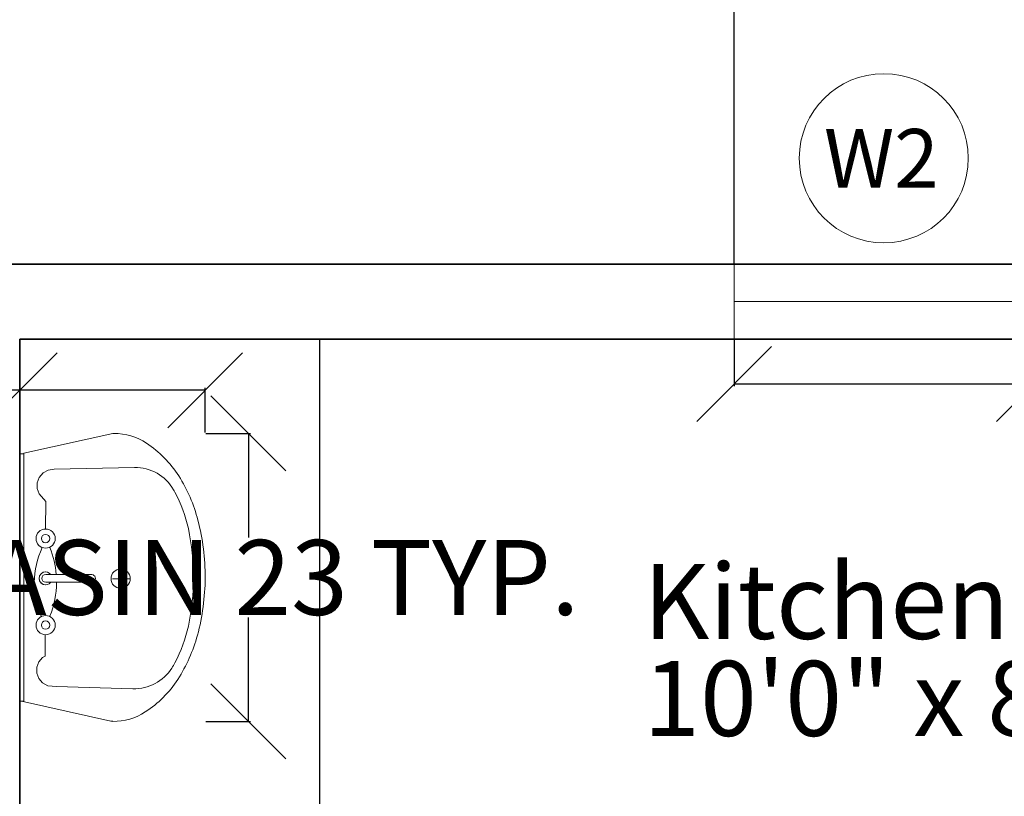
# Model space of a CAD drawing. Units: inches. Extents: x -1198 to -69, y -512 to 437.
# Tile 16 of 50: x -1013 to -934, y 221 to 283. Entities that reach past the tile are written whole.
import ezdxf

# ---------------------------------------------------------------- set-up
doc = ezdxf.new("R2010")
doc.units = ezdxf.units.IN
doc.header["$MEASUREMENT"] = 0
for name, color, linetype, lineweight in [('A-ANNO-DIMS', 2, 'Continuous', 18), ('A-ANNO-SYMB', 7, 'Continuous', 18), ('A-AREA-IDEN', 7, 'Continuous', 18), ('A-FLOR-CASE', 7, 'Continuous', 25), ('A-FLOR-FIXT', 60, 'Continuous', 18), ('A-WALL', 7, 'Continuous', 35), ('windows', 160, 'Continuous', 18)]:
    doc.layers.add(name, color=color, linetype=linetype, lineweight=lineweight)
doc.styles.get("Standard").update_dxf_attribs({"font": 'arial.ttf'})
doc.dimstyles.get("Standard").update_dxf_attribs({"dimtxt": 6, "dimasz": 6, "dimexe": 0.18, "dimexo": 0.0625, "dimgap": 0.09, "dimtad": 0, "dimtih": 1, "dimtoh": 1, "dimdec": 0, "dimzin": 0, "dimdsep": 46, "dimlunit": 4, "dimtxsty": 'Standard', "dimblk": 'OBLIQUE', "dimcen": 0.09, "dimadec": 0, "dimazin": 0, "dimtfac": 1, "dimtdec": 0, "dimtofl": 0, "dimtmove": 0, "dimatfit": 3, "dimfxl": 1, "dimtolj": 1, "dimtzin": 0, "dimarcsym": 0})

# ---------------------------------------------------------------- blocks, each defined once
blk = doc.blocks.new('A$C6AA41FE3')
at = {"linetype": 'ByBlock'}
for p, q in [((0.1919, 0.5849), (0.3733, 0.5439)), ((0.3687, 0.04), (0.3687, 0.5439)), ((0.3687, 0.5439), (0.3772, 0.5439)), ((0.3772, 0.0411), (0.3772, 0.5439)), ((0.3026, 0.514), (0.1469, 0.5187)), ((0.32, 0.5127), (0.3026, 0.514)), ((0.3305, 0.5069), (0.32, 0.5127)), ((0.3383, 0.4979), (0.3305, 0.5069)), ((0.3425, 0.4869), (0.3383, 0.4979)), ((0.3425, 0.4752), (0.3425, 0.4869)), ((0.3305, 0.4553), (0.3383, 0.4642)), ((0.3383, 0.4642), (0.3425, 0.4752)), ((0.3251, 0.409), (0.3253, 0.4524)), ((0.3253, 0.4524), (0.3305, 0.4553)), ((0.1747, 0.3146), (0.1747, 0.2774)), ((0.2326, 0.3025), (0.3243, 0.3025)), ((0.2326, 0.3021), (0.2326, 0.3025)), ((0.3243, 0.3025), (0.3243, 0.3024)), ((0.1525, 0.2951), (0.1884, 0.2951)), ((0.2326, 0.2863), (0.2326, 0.2867)), ((0.3243, 0.2863), (0.2326, 0.2863)), ((0.3243, 0.2864), (0.3243, 0.2863)), ((0.3243, 0.1379), (0.3245, 0.1941)), ((0.3374, 0.1229), (0.3243, 0.1379)), ((0.3415, 0.1119), (0.3374, 0.1229)), ((0.3374, 0.0892), (0.3415, 0.1002)), ((0.3415, 0.1002), (0.3415, 0.1119)), ((0.3191, 0.0744), (0.3296, 0.0802)), ((0.3296, 0.0802), (0.3374, 0.0892)), ((0.144, 0.0693), (0.3071, 0.0724)), ((0.3071, 0.0724), (0.3191, 0.0744)), ((0.3772, 0.0411), (0.3687, 0.0411)), ((0.188, 0), (0.3687, 0.04))]:
    blk.add_line(p, q, dxfattribs=at)
for centre, radius in [((0.3245, 0.3895), 0.0195), ((0.3245, 0.3895), 0.00849), ((0.172, 0.2951), 0.0195), ((0.3245, 0.2136), 0.0195), ((0.3245, 0.2136), 0.00849)]:
    blk.add_circle(centre, radius, dxfattribs=at)
for centre, radius, start, end in [((0.1864, 0.4671), 0.118, 89.1785, 123.1413), ((0.1877, 0.4667), 0.1183, 87.9266, 89.8113), ((0.241, 0.3799), 0.2208, 122.6461, 147.0936), ((0.1441, 0.4288), 0.09, 88.2595, 147.7588), ((0.3304, 0.324), 0.3262, 147.383, 164.6821), ((0.3272, 0.3256), 0.3003, 152.1306, 167.3001), ((0.2193, 0.3814), 0.1789, 147.7588, 151.7723), ((0.4743, 0.289), 0.4743, 165.1956, 179.4863), ((0.5, 0.2906), 0.4766, 167.7656, 179.7702), ((0.4839, 0.3016), 0.1818, 157.4645, 179.7061), ((0.1798, 0.3042), 0.1678, 334.4875, 24.1794), ((0.2312, 0.2944), 0.0078, 80.1551, 279.8449), ((0.3243, 0.2944), 0.013, 218.4979, 141.5021), ((0.3243, 0.2944), 0.0134, 270, 90), ((0.3243, 0.2944), 0.00798, 270, 90), ((0.4743, 0.2935), 0.4743, 180.0316, 194.3223), ((0.5, 0.2944), 0.4766, 180.2298, 192.2344), ((0.4839, 0.3016), 0.1818, 184.8087, 202.5355), ((0.3272, 0.2594), 0.3003, 192.6999, 207.8694), ((0.33, 0.2597), 0.3262, 194.841, 212.14), ((0.2193, 0.2037), 0.1789, 208.2281, 209.9799), ((0.1423, 0.1592), 0.09, 209.9799, 271.0537), ((0.2402, 0.2046), 0.2208, 212.4413, 236.8887), ((0.1848, 0.1179), 0.1179, 236.4084, 270.3713), ((0.1861, 0.1183), 0.1183, 269.7541, 270.9471)]:
    blk.add_arc(centre, radius, start, end, dxfattribs=at)
blk = doc.blocks.new('A1')
at = {"xscale": 1000, "yscale": 1000, "zscale": 1000, "rotation": 90}
blk.add_blockref('A$C6AA41FE3', (292.5, -377.2), dxfattribs=at)
blk = doc.blocks.new('WIN-W2-24')
at = {"ltscale": 10}
for p, q in [((0, 6), (0, 0)), ((24, 6), (24, 0)), ((0, 3), (24, 3))]:
    blk.add_line(p, q, dxfattribs=at)
blk = doc.blocks.new('COUNTER-L')
at = {"ltscale": 10}
for p, q in [((0, 96), (0, 24)), ((49.349, 24), (0, 24)), ((49.349, 0), (49.349, 24))]:
    blk.add_line(p, q, dxfattribs=at)
blk = doc.blocks.new('TAG-W2')
at = {"ltscale": 10}
blk.add_circle((0, 0), 6.767, dxfattribs=at)
blk.add_text('W2', height=4.6996, dxfattribs=at).set_placement((-4.791, -2.359))
blk = doc.blocks.new('_Oblique')
at = {"color": 0, "linetype": 'ByBlock', "lineweight": -2}
blk.add_line((-0.5, -0.5), (0.5, 0.5), dxfattribs=at)
blk = doc.blocks.new('*D40')
at = {"layer": 'A-ANNO-DIMS', "color": 0, "lineweight": -2, "ltscale": 10, "transparency": 16777216}
for p, q in [((-997.84, 249.671), (-994.265, 249.671)), ((-994.445, 249.671), (-994.445, 241.34)), ((-994.445, 226.62), (-994.445, 234.951)), ((-997.84, 226.62), (-994.265, 226.62))]:
    blk.add_line(p, q, dxfattribs=at)
at = {"layer": 'DEFPOINTS', "color": 0, "ltscale": 10, "transparency": 16777216}
for p in [(-997.902, 249.671), (-994.445, 249.671), (-997.902, 226.62)]:
    blk.add_point(p, dxfattribs=at)
at = {"layer": 'A-ANNO-DIMS', "color": 0, "lineweight": -2, "ltscale": 10, "transparency": 16777216, "xscale": 6, "yscale": 6, "zscale": 6}
for p, rotation in [((-994.445, 249.671), 90), ((-994.445, 226.62), 270)]:
    blk.add_blockref('_Oblique', p, dxfattribs=dict(at, rotation=rotation))
at = {"layer": 'A-ANNO-DIMS', "color": 0, "ltscale": 10, "transparency": 16777216, "insert": (-994.445, 238.145), "char_height": 6, "attachment_point": 5}
blk.add_mtext('\\A1;BASIN 23 TYP.', dxfattribs=at)
blk = doc.blocks.new('*D41')
at = {"layer": 'A-ANNO-DIMS', "color": 0, "lineweight": -2, "ltscale": 10, "transparency": 16777216}
for p, q in [((-1012.751, 253.128), (-1018.751, 253.128)), ((-1012.751, 249.733), (-1012.751, 253.308)), ((-997.902, 253.128), (-1012.751, 253.128)), ((-997.902, 249.733), (-997.902, 253.308))]:
    blk.add_line(p, q, dxfattribs=at)
at = {"layer": 'DEFPOINTS', "color": 0, "ltscale": 10, "transparency": 16777216}
for p in [(-1012.751, 253.128), (-1012.751, 249.671), (-997.902, 249.671)]:
    blk.add_point(p, dxfattribs=at)
at = {"layer": 'A-ANNO-DIMS', "color": 0, "lineweight": -2, "ltscale": 10, "transparency": 16777216, "xscale": 6, "yscale": 6, "zscale": 6, "rotation": 180}
blk.add_blockref('_Oblique', (-1012.751, 253.128), dxfattribs=at)
at = {"layer": 'A-ANNO-DIMS', "color": 0, "lineweight": -2, "ltscale": 10, "transparency": 16777216, "xscale": 6, "yscale": 6, "zscale": 6}
blk.add_blockref('_Oblique', (-997.902, 253.128), dxfattribs=at)
at = {"layer": 'A-ANNO-DIMS', "color": 0, "ltscale": 10, "transparency": 16777216, "insert": (-1033.161, 253.128), "char_height": 6, "attachment_point": 5}
blk.add_mtext('\\A1;15 TYP.', dxfattribs=at)
blk = doc.blocks.new('*D48')
at = {"layer": 'A-ANNO-DIMS', "color": 0, "lineweight": -2, "ltscale": 10, "transparency": 16777216}
for p, q in [((-955.559, 257.165), (-955.559, 253.448)), ((-931.559, 257.165), (-931.559, 253.448)), ((-955.559, 253.628), (-931.559, 253.628)), ((-931.559, 253.628), (-925.559, 253.628))]:
    blk.add_line(p, q, dxfattribs=at)
at = {"layer": 'DEFPOINTS', "color": 0, "ltscale": 10, "transparency": 16777216}
for p in [(-955.559, 257.228), (-931.559, 257.228), (-931.559, 253.628)]:
    blk.add_point(p, dxfattribs=at)
at = {"layer": 'A-ANNO-DIMS', "color": 0, "lineweight": -2, "ltscale": 10, "transparency": 16777216, "xscale": 6, "yscale": 6, "zscale": 6, "rotation": 180}
blk.add_blockref('_Oblique', (-955.559, 253.628), dxfattribs=at)
at = {"layer": 'A-ANNO-DIMS', "color": 0, "lineweight": -2, "ltscale": 10, "transparency": 16777216, "xscale": 6, "yscale": 6, "zscale": 6}
blk.add_blockref('_Oblique', (-931.559, 253.628), dxfattribs=at)
at = {"layer": 'A-ANNO-DIMS', "color": 0, "ltscale": 10, "transparency": 16777216, "insert": (-903.292, 253.628), "char_height": 6, "attachment_point": 5}
blk.add_mtext('\\A1;W2 24 TYP.', dxfattribs=at)
blk = doc.blocks.new('*D78')
at = {"layer": 'A-ANNO-DIMS', "color": 0, "lineweight": -2, "ltscale": 10, "transparency": 16777216}
for p, q in [((-1018.751, 263.29), (-1018.751, 433.184)), ((-1018.751, 433.004), (-997.391, 433.004)), ((-955.559, 433.004), (-976.919, 433.004)), ((-955.559, 263.29), (-955.559, 433.184))]:
    blk.add_line(p, q, dxfattribs=at)
at = {"layer": 'DEFPOINTS', "color": 0, "ltscale": 10, "transparency": 16777216}
for p in [(-955.559, 433.004), (-1018.751, 263.228), (-955.559, 263.228)]:
    blk.add_point(p, dxfattribs=at)
at = {"layer": 'A-ANNO-DIMS', "color": 0, "lineweight": -2, "ltscale": 10, "transparency": 16777216, "xscale": 6, "yscale": 6, "zscale": 6, "rotation": 180}
blk.add_blockref('_Oblique', (-1018.751, 433.004), dxfattribs=at)
at = {"layer": 'A-ANNO-DIMS', "color": 0, "lineweight": -2, "ltscale": 10, "transparency": 16777216, "xscale": 6, "yscale": 6, "zscale": 6}
blk.add_blockref('_Oblique', (-955.559, 433.004), dxfattribs=at)
at = {"layer": 'A-ANNO-DIMS', "color": 0, "ltscale": 10, "transparency": 16777216, "insert": (-987.155, 433.004), "char_height": 6, "attachment_point": 5}
blk.add_mtext('\\A1;63.19', dxfattribs=at)

msp = doc.modelspace()

# ---------------------------------------------------------------- linework, layer by layer
at = {"layer": 'A-WALL', "ltscale": 10}
for p, q in [((-697.7509, 263.2277), (-1018.7509, 263.2277)), ((-1012.7509, 257.2277), (-1012.7509, 161.2277)), ((-1012.7509, 257.2277), (-922.6458, 257.2277))]:
    msp.add_line(p, q, dxfattribs=at)

# ---------------------------------------------------------------- block references
at = {"layer": 'A-ANNO-SYMB'}
msp.add_blockref('TAG-W2', (-943.5812, 271.6962), dxfattribs=at)
at = {"layer": 'A-FLOR-CASE'}
msp.add_blockref('COUNTER-L', (-988.751, 161.228), dxfattribs=at)
at = {"layer": 'A-FLOR-FIXT', "ltscale": 10, "xscale": 0.0393700787401575, "yscale": 0.0393700787401575, "zscale": 0.0393700787401575, "rotation": 90}
msp.add_blockref('A1', (-1012.7509, 238.1491), dxfattribs=at)
at = {"layer": 'windows'}
msp.add_blockref('WIN-W2-24', (-955.559, 257.228), dxfattribs=at)

# ---------------------------------------------------------------- texts
at = {"layer": 'A-AREA-IDEN', "ltscale": 10, "char_height": 6, "attachment_point": 1}
for s, insert in [('Kitchen', (-962.8292, 239.2277)), ('10\'0" x 8\'0"', (-962.8292, 231.4637))]:
    msp.add_mtext_dynamic_manual_height_columns(s, width=57.976527, gutter_width=30, heights=[0], dxfattribs=dict(at, insert=insert))

# ---------------------------------------------------------------- dimensions: what is measured, and where the dimension line sits
at = {"layer": 'A-ANNO-DIMS', "ltscale": 10}
dim = msp.add_linear_dim(base=(-955.5591, 433.0036), p1=(-1018.7509, 263.2277), p2=(-955.5591, 263.2277), dimstyle='Standard', override={"dimdec": 2, "dimlfac": 1, "dimrnd": 0, "dimzin": 0, "dimdsep": 46, "dimlunit": 2}, dxfattribs=at)
dim.commit()
dim.dimension.update_dxf_attribs({"geometry": '*D78', "text_midpoint": (-987.155, 433.0036)})
dim = msp.add_linear_dim(base=(-931.5591, 253.6277), p1=(-955.5591, 257.2277), p2=(-931.5591, 257.2277), text='W2 <> TYP.', dimstyle='Standard', override={"dimdec": 0, "dimlfac": 1, "dimrnd": 0, "dimzin": 0, "dimdsep": 46, "dimlunit": 2}, dxfattribs=at)
dim.commit()
dim.dimension.update_dxf_attribs({"geometry": '*D48', "text_midpoint": (-903.2925, 253.6277)})
for base, p1, p2, angle, text, picture, middle in [((-1012.7509, 253.1284), (-997.9022, 249.6708), (-1012.7509, 249.6708), 180, '<> TYP.', '*D41', (-1033.1615, 253.1284)), ((-994.4446, 249.6708), (-997.9022, 226.6201), (-997.9022, 249.6708), 90, 'BASIN <> TYP.', '*D40', (-994.4446, 238.1454))]:
    dim = msp.add_linear_dim(base=base, p1=p1, p2=p2, angle=angle, text=text, dimstyle='Standard', override={"dimdec": 0, "dimlfac": 1, "dimrnd": 0, "dimzin": 0, "dimdsep": 46, "dimlunit": 2}, dxfattribs=at)
    dim.commit()
    dim.dimension.update_dxf_attribs({"geometry": picture, "text_midpoint": middle})

doc.saveas('drawing.dxf')
